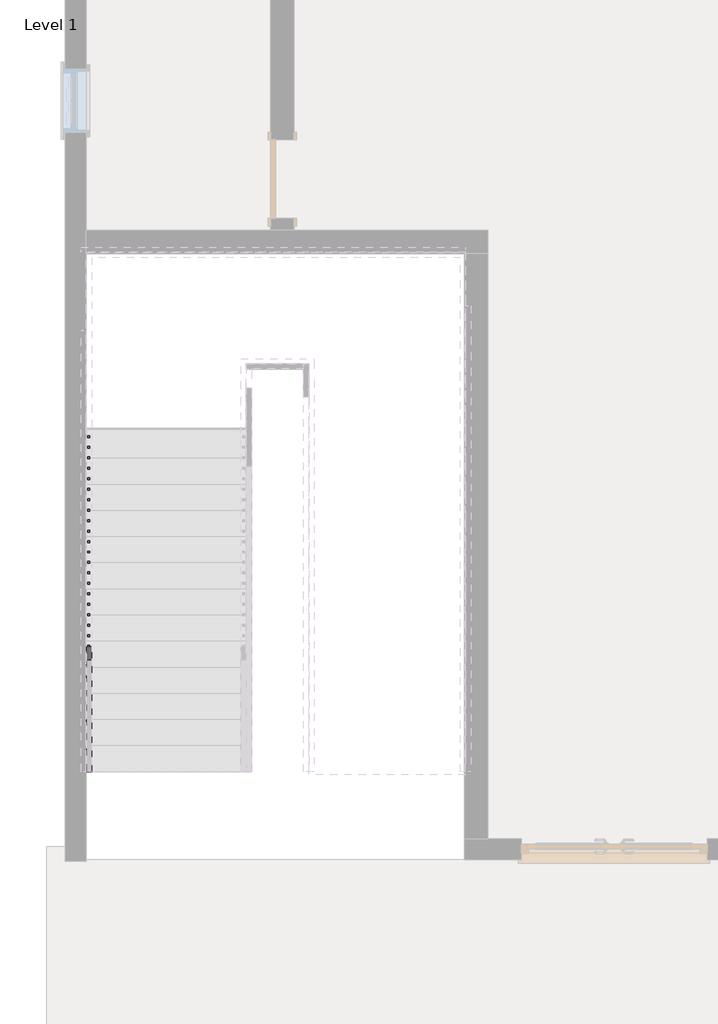
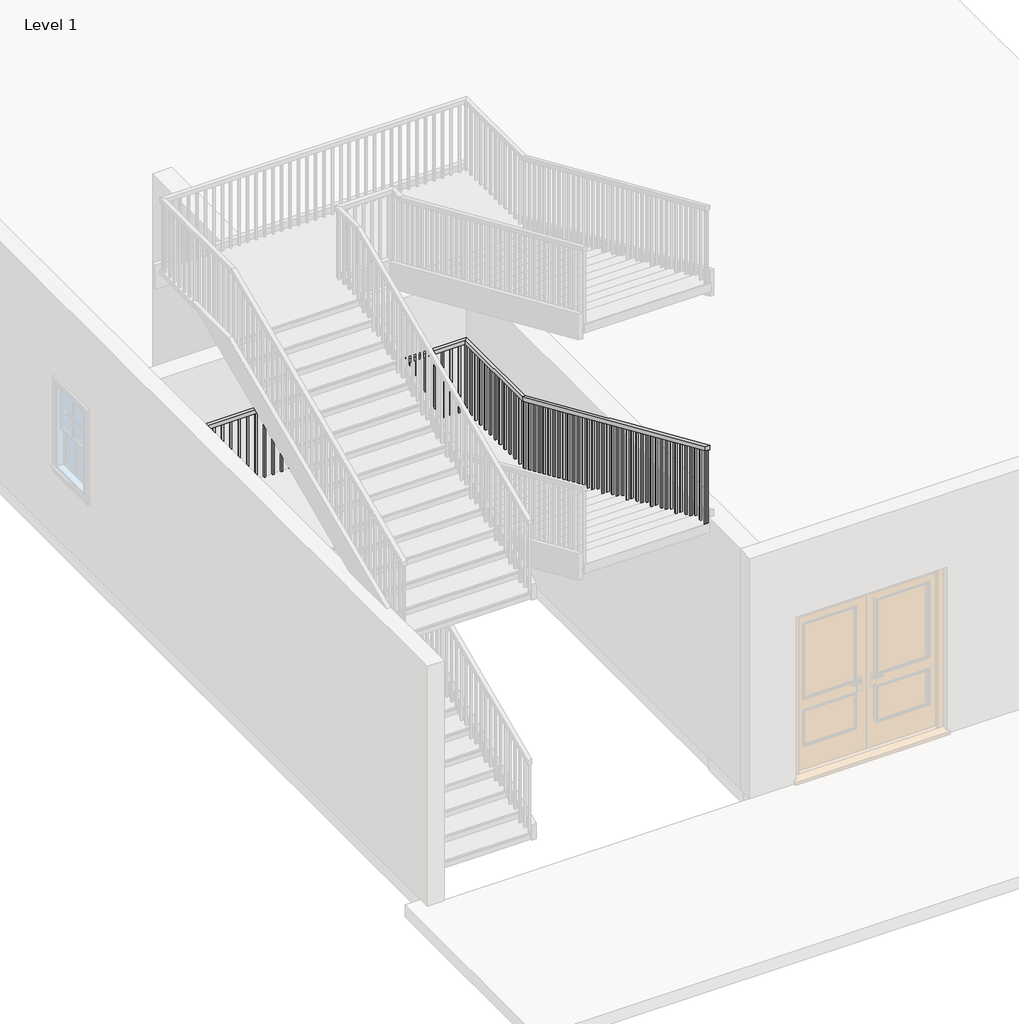
# One storey, part 3 of 6: 1 railing.
"""IFC4 building model written with IfcOpenShell, lengths in millimetres."""

from ifc_helpers import new_model, si_unit, frame, origin, place, context, project, spatial, polyline, outline, extrude, faceted_brep, element, save

model = new_model("IFC4")

# Units and contexts
model_context = context("Model", 3, world=origin())
ifc_project = project(units=[si_unit("LENGTHUNIT", "METRE", prefix="MILLI")], contexts=[model_context])

# Site, building, storey
site = spatial("IfcSite", under=ifc_project)
building = spatial("IfcBuilding", under=site)
storey = spatial("IfcBuildingStorey", under=building, Name="Level 1", Elevation=0.0)

# Railing
placement = place(None, origin())
element("IfcRailing", 1, ObjectType="Handrail - Rectangular", at=placement, inside=storey, context=model_context, shape_type="SolidModel", body=[
    faceted_brep([(-7554.4415084, -6973.0610642, 721.36), (-7554.4415084, -6973.0610642, 665.8599828), (-7503.6415084, -6973.0610642, 665.8599828), (-7503.6415084, -6973.0610642, 721.36), (-7554.4415084, -3417.0610642, 2286.0), (-7554.4415084, -3406.3792071, 2235.2), (-7503.6415084, -3406.3792071, 2235.2), (-7503.6415084, -3417.0610642, 2286.0), (-7554.4415084, -1928.4217109, 2286.0), (-7554.4415084, -1928.4217109, 2235.2), (-7503.6415084, -1979.2217109, 2235.2), (-7503.6415084, -1979.2217109, 2286.0), (-3866.3290366, -1928.4217109, 2286.0), (-3866.3290366, -1928.4217109, 2235.2), (-3917.1290366, -1979.2217109, 2235.2), (-3917.1290366, -1979.2217109, 2286.0), (-3866.3290366, -3163.0610642, 2286.0), (-3866.3290366, -3173.7429214, 2235.2), (-3917.1290366, -3173.7429214, 2235.2), (-3917.1290366, -3163.0610642, 2286.0), (-3866.3290366, -6973.0610642, 3962.4), (-3917.1290366, -6973.0610642, 3962.4), (-3917.1290366, -6973.0610642, 3906.8999828), (-3866.3290366, -6973.0610642, 3906.8999828)], [[[0, 1, 2, 3]], [[1, 0, 4, 5]], [[2, 1, 5, 6]], [[3, 2, 6, 7]], [[0, 3, 7, 4]], [[5, 4, 8, 9]], [[6, 5, 9, 10]], [[7, 6, 10, 11]], [[4, 7, 11, 8]], [[9, 8, 12, 13]], [[10, 9, 13, 14]], [[11, 10, 14, 15]], [[8, 11, 15, 12]], [[13, 12, 16, 17]], [[14, 13, 17, 18]], [[15, 14, 18, 19]], [[12, 15, 19, 16]], [[20, 21, 22, 23]], [[17, 16, 20, 23]], [[18, 17, 23, 22]], [[19, 18, 22, 21]], [[16, 19, 21, 20]]]),
    extrude(outline(polyline([(-6922.6967109, 3884.7396674), (-6922.6967109, 2936.24), (-6941.7467109, 2936.24), (-6941.7467109, 3893.1216674), (-6922.6967109, 3884.7396674)])), frame((-3901.2540366, 0.0, 0.0), z_axis=(1.0, 0.0, 0.0), x_axis=(0.0, 1.0, 0.0)), (0.0, 0.0, 1.0), 19.05),
    extrude(outline(polyline([(-6821.0967109, 3840.0356674), (-6821.0967109, 2936.24), (-6840.1467109, 2936.24), (-6840.1467109, 3848.4176674), (-6821.0967109, 3840.0356674)])), frame((-3901.2540366, 0.0, 0.0), z_axis=(1.0, 0.0, 0.0), x_axis=(0.0, 1.0, 0.0)), (0.0, 0.0, 1.0), 19.05),
    extrude(outline(polyline([(-6719.4967109, 3795.3316674), (-6719.4967109, 2936.24), (-6738.5467109, 2936.24), (-6738.5467109, 3803.7136674), (-6719.4967109, 3795.3316674)])), frame((-3901.2540366, 0.0, 0.0), z_axis=(1.0, 0.0, 0.0), x_axis=(0.0, 1.0, 0.0)), (0.0, 0.0, 1.0), 19.05),
    extrude(outline(polyline([(-6617.8967109, 3750.6276674), (-6617.8967109, 2824.48), (-6636.9467109, 2824.48), (-6636.9467109, 3759.0096674), (-6617.8967109, 3750.6276674)])), frame((-3901.2540366, 0.0, 0.0), z_axis=(1.0, 0.0, 0.0), x_axis=(0.0, 1.0, 0.0)), (0.0, 0.0, 1.0), 19.05),
    extrude(outline(polyline([(-6516.2967109, 3705.9236674), (-6516.2967109, 2824.48), (-6535.3467109, 2824.48), (-6535.3467109, 3714.3056674), (-6516.2967109, 3705.9236674)])), frame((-3901.2540366, 0.0, 0.0), z_axis=(1.0, 0.0, 0.0), x_axis=(0.0, 1.0, 0.0)), (0.0, 0.0, 1.0), 19.05),
    extrude(outline(polyline([(-6414.6967109, 3661.2196674), (-6414.6967109, 2712.72), (-6433.7467109, 2712.72), (-6433.7467109, 3669.6016674), (-6414.6967109, 3661.2196674)])), frame((-3901.2540366, 0.0, 0.0), z_axis=(1.0, 0.0, 0.0), x_axis=(0.0, 1.0, 0.0)), (0.0, 0.0, 1.0), 19.05),
    extrude(outline(polyline([(-6313.0967109, 3616.5156674), (-6313.0967109, 2712.72), (-6332.1467109, 2712.72), (-6332.1467109, 3624.8976674), (-6313.0967109, 3616.5156674)])), frame((-3901.2540366, 0.0, 0.0), z_axis=(1.0, 0.0, 0.0), x_axis=(0.0, 1.0, 0.0)), (0.0, 0.0, 1.0), 19.05),
    extrude(outline(polyline([(-6211.4967109, 3571.8116674), (-6211.4967109, 2712.72), (-6230.5467109, 2712.72), (-6230.5467109, 3580.1936674), (-6211.4967109, 3571.8116674)])), frame((-3901.2540366, 0.0, 0.0), z_axis=(1.0, 0.0, 0.0), x_axis=(0.0, 1.0, 0.0)), (0.0, 0.0, 1.0), 19.05),
    extrude(outline(polyline([(-6109.8967109, 3527.1076674), (-6109.8967109, 2600.96), (-6128.9467109, 2600.96), (-6128.9467109, 3535.4896674), (-6109.8967109, 3527.1076674)])), frame((-3901.2540366, 0.0, 0.0), z_axis=(1.0, 0.0, 0.0), x_axis=(0.0, 1.0, 0.0)), (0.0, 0.0, 1.0), 19.05),
    extrude(outline(polyline([(-6008.2967109, 3482.4036674), (-6008.2967109, 2600.96), (-6027.3467109, 2600.96), (-6027.3467109, 3490.7856674), (-6008.2967109, 3482.4036674)])), frame((-3901.2540366, 0.0, 0.0), z_axis=(1.0, 0.0, 0.0), x_axis=(0.0, 1.0, 0.0)), (0.0, 0.0, 1.0), 19.05),
    extrude(outline(polyline([(-5906.6967109, 3437.6996674), (-5906.6967109, 2489.2), (-5925.7467109, 2489.2), (-5925.7467109, 3446.0816674), (-5906.6967109, 3437.6996674)])), frame((-3901.2540366, 0.0, 0.0), z_axis=(1.0, 0.0, 0.0), x_axis=(0.0, 1.0, 0.0)), (0.0, 0.0, 1.0), 19.05),
    extrude(outline(polyline([(-5805.0967109, 3392.9956674), (-5805.0967109, 2489.2), (-5824.1467109, 2489.2), (-5824.1467109, 3401.3776674), (-5805.0967109, 3392.9956674)])), frame((-3901.2540366, 0.0, 0.0), z_axis=(1.0, 0.0, 0.0), x_axis=(0.0, 1.0, 0.0)), (0.0, 0.0, 1.0), 19.05),
    extrude(outline(polyline([(-5703.4967109, 3348.2916674), (-5703.4967109, 2489.2), (-5722.5467109, 2489.2), (-5722.5467109, 3356.6736674), (-5703.4967109, 3348.2916674)])), frame((-3901.2540366, 0.0, 0.0), z_axis=(1.0, 0.0, 0.0), x_axis=(0.0, 1.0, 0.0)), (0.0, 0.0, 1.0), 19.05),
    extrude(outline(polyline([(-5601.8967109, 3303.5876674), (-5601.8967109, 2377.44), (-5620.9467109, 2377.44), (-5620.9467109, 3311.9696674), (-5601.8967109, 3303.5876674)])), frame((-3901.2540366, 0.0, 0.0), z_axis=(1.0, 0.0, 0.0), x_axis=(0.0, 1.0, 0.0)), (0.0, 0.0, 1.0), 19.05),
    extrude(outline(polyline([(-5500.2967109, 3258.8836674), (-5500.2967109, 2377.44), (-5519.3467109, 2377.44), (-5519.3467109, 3267.2656674), (-5500.2967109, 3258.8836674)])), frame((-3901.2540366, 0.0, 0.0), z_axis=(1.0, 0.0, 0.0), x_axis=(0.0, 1.0, 0.0)), (0.0, 0.0, 1.0), 19.05),
    extrude(outline(polyline([(-5398.6967109, 3214.1796674), (-5398.6967109, 2265.68), (-5417.7467109, 2265.68), (-5417.7467109, 3222.5616674), (-5398.6967109, 3214.1796674)])), frame((-3901.2540366, 0.0, 0.0), z_axis=(1.0, 0.0, 0.0), x_axis=(0.0, 1.0, 0.0)), (0.0, 0.0, 1.0), 19.05),
    extrude(outline(polyline([(-5297.0967109, 3169.4756674), (-5297.0967109, 2265.68), (-5316.1467109, 2265.68), (-5316.1467109, 3177.8576674), (-5297.0967109, 3169.4756674)])), frame((-3901.2540366, 0.0, 0.0), z_axis=(1.0, 0.0, 0.0), x_axis=(0.0, 1.0, 0.0)), (0.0, 0.0, 1.0), 19.05),
    extrude(outline(polyline([(-5195.4967109, 3124.7716674), (-5195.4967109, 2265.68), (-5214.5467109, 2265.68), (-5214.5467109, 3133.1536674), (-5195.4967109, 3124.7716674)])), frame((-3901.2540366, 0.0, 0.0), z_axis=(1.0, 0.0, 0.0), x_axis=(0.0, 1.0, 0.0)), (0.0, 0.0, 1.0), 19.05),
    extrude(outline(polyline([(-5093.8967109, 3080.0676674), (-5093.8967109, 2153.92), (-5112.9467109, 2153.92), (-5112.9467109, 3088.4496674), (-5093.8967109, 3080.0676674)])), frame((-3901.2540366, 0.0, 0.0), z_axis=(1.0, 0.0, 0.0), x_axis=(0.0, 1.0, 0.0)), (0.0, 0.0, 1.0), 19.05),
    extrude(outline(polyline([(-4992.2967109, 3035.3636674), (-4992.2967109, 2153.92), (-5011.3467109, 2153.92), (-5011.3467109, 3043.7456674), (-4992.2967109, 3035.3636674)])), frame((-3901.2540366, 0.0, 0.0), z_axis=(1.0, 0.0, 0.0), x_axis=(0.0, 1.0, 0.0)), (0.0, 0.0, 1.0), 19.05),
    extrude(outline(polyline([(-4890.6967109, 2990.6596674), (-4890.6967109, 2042.16), (-4909.7467109, 2042.16), (-4909.7467109, 2999.0416674), (-4890.6967109, 2990.6596674)])), frame((-3901.2540366, 0.0, 0.0), z_axis=(1.0, 0.0, 0.0), x_axis=(0.0, 1.0, 0.0)), (0.0, 0.0, 1.0), 19.05),
    extrude(outline(polyline([(-4789.0967109, 2945.9556674), (-4789.0967109, 2042.16), (-4808.1467109, 2042.16), (-4808.1467109, 2954.3376674), (-4789.0967109, 2945.9556674)])), frame((-3901.2540366, 0.0, 0.0), z_axis=(1.0, 0.0, 0.0), x_axis=(0.0, 1.0, 0.0)), (0.0, 0.0, 1.0), 19.05),
    extrude(outline(polyline([(-4687.4967109, 2901.2516674), (-4687.4967109, 2042.16), (-4706.5467109, 2042.16), (-4706.5467109, 2909.6336674), (-4687.4967109, 2901.2516674)])), frame((-3901.2540366, 0.0, 0.0), z_axis=(1.0, 0.0, 0.0), x_axis=(0.0, 1.0, 0.0)), (0.0, 0.0, 1.0), 19.05),
    extrude(outline(polyline([(-4585.8967109, 2856.5476674), (-4585.8967109, 1930.4), (-4604.9467109, 1930.4), (-4604.9467109, 2864.9296674), (-4585.8967109, 2856.5476674)])), frame((-3901.2540366, 0.0, 0.0), z_axis=(1.0, 0.0, 0.0), x_axis=(0.0, 1.0, 0.0)), (0.0, 0.0, 1.0), 19.05),
    extrude(outline(polyline([(-4484.2967109, 2811.8436674), (-4484.2967109, 1930.4), (-4503.3467109, 1930.4), (-4503.3467109, 2820.2256674), (-4484.2967109, 2811.8436674)])), frame((-3901.2540366, 0.0, 0.0), z_axis=(1.0, 0.0, 0.0), x_axis=(0.0, 1.0, 0.0)), (0.0, 0.0, 1.0), 19.05),
    extrude(outline(polyline([(-4382.6967109, 2767.1396674), (-4382.6967109, 1818.64), (-4401.7467109, 1818.64), (-4401.7467109, 2775.5216674), (-4382.6967109, 2767.1396674)])), frame((-3901.2540366, 0.0, 0.0), z_axis=(1.0, 0.0, 0.0), x_axis=(0.0, 1.0, 0.0)), (0.0, 0.0, 1.0), 19.05),
    extrude(outline(polyline([(-4281.0967109, 2722.4356674), (-4281.0967109, 1818.64), (-4300.1467109, 1818.64), (-4300.1467109, 2730.8176674), (-4281.0967109, 2722.4356674)])), frame((-3901.2540366, 0.0, 0.0), z_axis=(1.0, 0.0, 0.0), x_axis=(0.0, 1.0, 0.0)), (0.0, 0.0, 1.0), 19.05),
    extrude(outline(polyline([(-4179.4967109, 2677.7316674), (-4179.4967109, 1818.64), (-4198.5467109, 1818.64), (-4198.5467109, 2686.1136674), (-4179.4967109, 2677.7316674)])), frame((-3901.2540366, 0.0, 0.0), z_axis=(1.0, 0.0, 0.0), x_axis=(0.0, 1.0, 0.0)), (0.0, 0.0, 1.0), 19.05),
    extrude(outline(polyline([(-4077.8967109, 2633.0276674), (-4077.8967109, 1706.88), (-4096.9467109, 1706.88), (-4096.9467109, 2641.4096674), (-4077.8967109, 2633.0276674)])), frame((-3901.2540366, 0.0, 0.0), z_axis=(1.0, 0.0, 0.0), x_axis=(0.0, 1.0, 0.0)), (0.0, 0.0, 1.0), 19.05),
    extrude(outline(polyline([(-3976.2967109, 2588.3236674), (-3976.2967109, 1706.88), (-3995.3467109, 1706.88), (-3995.3467109, 2596.7056674), (-3976.2967109, 2588.3236674)])), frame((-3901.2540366, 0.0, 0.0), z_axis=(1.0, 0.0, 0.0), x_axis=(0.0, 1.0, 0.0)), (0.0, 0.0, 1.0), 19.05),
    extrude(outline(polyline([(-3874.6967109, 2543.6196674), (-3874.6967109, 1595.12), (-3893.7467109, 1595.12), (-3893.7467109, 2552.0016674), (-3874.6967109, 2543.6196674)])), frame((-3901.2540366, 0.0, 0.0), z_axis=(1.0, 0.0, 0.0), x_axis=(0.0, 1.0, 0.0)), (0.0, 0.0, 1.0), 19.05),
    extrude(outline(polyline([(-3773.0967109, 2498.9156674), (-3773.0967109, 1595.12), (-3792.1467109, 1595.12), (-3792.1467109, 2507.2976674), (-3773.0967109, 2498.9156674)])), frame((-3901.2540366, 0.0, 0.0), z_axis=(1.0, 0.0, 0.0), x_axis=(0.0, 1.0, 0.0)), (0.0, 0.0, 1.0), 19.05),
    extrude(outline(polyline([(-3671.4967109, 2454.2116674), (-3671.4967109, 1595.12), (-3690.5467109, 1595.12), (-3690.5467109, 2462.5936674), (-3671.4967109, 2454.2116674)])), frame((-3901.2540366, 0.0, 0.0), z_axis=(1.0, 0.0, 0.0), x_axis=(0.0, 1.0, 0.0)), (0.0, 0.0, 1.0), 19.05),
    extrude(outline(polyline([(-3569.8967109, 2409.5076674), (-3569.8967109, 1483.36), (-3588.9467109, 1483.36), (-3588.9467109, 2417.8896674), (-3569.8967109, 2409.5076674)])), frame((-3901.2540366, 0.0, 0.0), z_axis=(1.0, 0.0, 0.0), x_axis=(0.0, 1.0, 0.0)), (0.0, 0.0, 1.0), 19.05),
    extrude(outline(polyline([(-3468.2967109, 2364.8036674), (-3468.2967109, 1483.36), (-3487.3467109, 1483.36), (-3487.3467109, 2373.1856674), (-3468.2967109, 2364.8036674)])), frame((-3901.2540366, 0.0, 0.0), z_axis=(1.0, 0.0, 0.0), x_axis=(0.0, 1.0, 0.0)), (0.0, 0.0, 1.0), 19.05),
    extrude(outline(polyline([(-3366.6967109, 2320.0996674), (-3366.6967109, 1371.6), (-3385.7467109, 1371.6), (-3385.7467109, 2328.4816674), (-3366.6967109, 2320.0996674)])), frame((-3901.2540366, 0.0, 0.0), z_axis=(1.0, 0.0, 0.0), x_axis=(0.0, 1.0, 0.0)), (0.0, 0.0, 1.0), 19.05),
    extrude(outline(polyline([(-3265.0967109, 2275.3956674), (-3265.0967109, 1371.6), (-3284.1467109, 1371.6), (-3284.1467109, 2283.7776674), (-3265.0967109, 2275.3956674)])), frame((-3901.2540366, 0.0, 0.0), z_axis=(1.0, 0.0, 0.0), x_axis=(0.0, 1.0, 0.0)), (0.0, 0.0, 1.0), 19.05),
    extrude(outline(polyline([(-3163.4967109, 2230.6916674), (-3163.4967109, 1371.6), (-3182.5467109, 1371.6), (-3182.5467109, 2239.0736674), (-3163.4967109, 2230.6916674)])), frame((-3901.2540366, 0.0, 0.0), z_axis=(1.0, 0.0, 0.0), x_axis=(0.0, 1.0, 0.0)), (0.0, 0.0, 1.0), 19.05),
    extrude(outline(polyline([(-3882.2040366, -3061.8967109), (-3882.2040366, -3080.9467109), (-3901.2540366, -3080.9467109), (-3901.2540366, -3061.8967109), (-3882.2040366, -3061.8967109)])), frame((0.0, 0.0, 1371.6), z_axis=(0.0, 0.0, 1.0), x_axis=(1.0, 0.0, 0.0)), (0.0, 0.0, 1.0), 863.6),
    extrude(outline(polyline([(-3882.2040366, -2960.2967109), (-3882.2040366, -2979.3467109), (-3901.2540366, -2979.3467109), (-3901.2540366, -2960.2967109), (-3882.2040366, -2960.2967109)])), frame((0.0, 0.0, 1371.6), z_axis=(0.0, 0.0, 1.0), x_axis=(1.0, 0.0, 0.0)), (0.0, 0.0, 1.0), 863.6),
    extrude(outline(polyline([(-3882.2040366, -2858.6967109), (-3882.2040366, -2877.7467109), (-3901.2540366, -2877.7467109), (-3901.2540366, -2858.6967109), (-3882.2040366, -2858.6967109)])), frame((0.0, 0.0, 1371.6), z_axis=(0.0, 0.0, 1.0), x_axis=(1.0, 0.0, 0.0)), (0.0, 0.0, 1.0), 863.6),
    extrude(outline(polyline([(-3882.2040366, -2757.0967109), (-3882.2040366, -2776.1467109), (-3901.2540366, -2776.1467109), (-3901.2540366, -2757.0967109), (-3882.2040366, -2757.0967109)])), frame((0.0, 0.0, 1371.6), z_axis=(0.0, 0.0, 1.0), x_axis=(1.0, 0.0, 0.0)), (0.0, 0.0, 1.0), 863.6),
    extrude(outline(polyline([(-3882.2040366, -2655.4967109), (-3882.2040366, -2674.5467109), (-3901.2540366, -2674.5467109), (-3901.2540366, -2655.4967109), (-3882.2040366, -2655.4967109)])), frame((0.0, 0.0, 1371.6), z_axis=(0.0, 0.0, 1.0), x_axis=(1.0, 0.0, 0.0)), (0.0, 0.0, 1.0), 863.6),
    extrude(outline(polyline([(-3882.2040366, -2553.8967109), (-3882.2040366, -2572.9467109), (-3901.2540366, -2572.9467109), (-3901.2540366, -2553.8967109), (-3882.2040366, -2553.8967109)])), frame((0.0, 0.0, 1371.6), z_axis=(0.0, 0.0, 1.0), x_axis=(1.0, 0.0, 0.0)), (0.0, 0.0, 1.0), 863.6),
    extrude(outline(polyline([(-3882.2040366, -2452.2967109), (-3882.2040366, -2471.3467109), (-3901.2540366, -2471.3467109), (-3901.2540366, -2452.2967109), (-3882.2040366, -2452.2967109)])), frame((0.0, 0.0, 1371.6), z_axis=(0.0, 0.0, 1.0), x_axis=(1.0, 0.0, 0.0)), (0.0, 0.0, 1.0), 863.6),
    extrude(outline(polyline([(-3882.2040366, -2350.6967109), (-3882.2040366, -2369.7467109), (-3901.2540366, -2369.7467109), (-3901.2540366, -2350.6967109), (-3882.2040366, -2350.6967109)])), frame((0.0, 0.0, 1371.6), z_axis=(0.0, 0.0, 1.0), x_axis=(1.0, 0.0, 0.0)), (0.0, 0.0, 1.0), 863.6),
    extrude(outline(polyline([(-3882.2040366, -2249.0967109), (-3882.2040366, -2268.1467109), (-3901.2540366, -2268.1467109), (-3901.2540366, -2249.0967109), (-3882.2040366, -2249.0967109)])), frame((0.0, 0.0, 1371.6), z_axis=(0.0, 0.0, 1.0), x_axis=(1.0, 0.0, 0.0)), (0.0, 0.0, 1.0), 863.6),
    extrude(outline(polyline([(-3882.2040366, -2147.4967109), (-3882.2040366, -2166.5467109), (-3901.2540366, -2166.5467109), (-3901.2540366, -2147.4967109), (-3882.2040366, -2147.4967109)])), frame((0.0, 0.0, 1371.6), z_axis=(0.0, 0.0, 1.0), x_axis=(1.0, 0.0, 0.0)), (0.0, 0.0, 1.0), 863.6),
    extrude(outline(polyline([(-3882.2040366, -2045.8967109), (-3882.2040366, -2064.9467109), (-3901.2540366, -2064.9467109), (-3901.2540366, -2045.8967109), (-3882.2040366, -2045.8967109)])), frame((0.0, 0.0, 1371.6), z_axis=(0.0, 0.0, 1.0), x_axis=(1.0, 0.0, 0.0)), (0.0, 0.0, 1.0), 863.6),
    extrude(outline(polyline([(-3982.5665084, -1944.2967109), (-3963.5165084, -1944.2967109), (-3963.5165084, -1963.3467109), (-3982.5665084, -1963.3467109), (-3982.5665084, -1944.2967109)])), frame((0.0, 0.0, 1371.6), z_axis=(0.0, 0.0, 1.0), x_axis=(1.0, 0.0, 0.0)), (0.0, 0.0, 1.0), 863.6),
    extrude(outline(polyline([(-4084.1665084, -1944.2967109), (-4065.1165084, -1944.2967109), (-4065.1165084, -1963.3467109), (-4084.1665084, -1963.3467109), (-4084.1665084, -1944.2967109)])), frame((0.0, 0.0, 1371.6), z_axis=(0.0, 0.0, 1.0), x_axis=(1.0, 0.0, 0.0)), (0.0, 0.0, 1.0), 863.6),
    extrude(outline(polyline([(-4185.7665084, -1944.2967109), (-4166.7165084, -1944.2967109), (-4166.7165084, -1963.3467109), (-4185.7665084, -1963.3467109), (-4185.7665084, -1944.2967109)])), frame((0.0, 0.0, 1371.6), z_axis=(0.0, 0.0, 1.0), x_axis=(1.0, 0.0, 0.0)), (0.0, 0.0, 1.0), 863.6),
    extrude(outline(polyline([(-4287.3665084, -1944.2967109), (-4268.3165084, -1944.2967109), (-4268.3165084, -1963.3467109), (-4287.3665084, -1963.3467109), (-4287.3665084, -1944.2967109)])), frame((0.0, 0.0, 1371.6), z_axis=(0.0, 0.0, 1.0), x_axis=(1.0, 0.0, 0.0)), (0.0, 0.0, 1.0), 863.6),
    extrude(outline(polyline([(-4388.9665084, -1944.2967109), (-4369.9165084, -1944.2967109), (-4369.9165084, -1963.3467109), (-4388.9665084, -1963.3467109), (-4388.9665084, -1944.2967109)])), frame((0.0, 0.0, 1371.6), z_axis=(0.0, 0.0, 1.0), x_axis=(1.0, 0.0, 0.0)), (0.0, 0.0, 1.0), 863.6),
    extrude(outline(polyline([(-4490.5665084, -1944.2967109), (-4471.5165084, -1944.2967109), (-4471.5165084, -1963.3467109), (-4490.5665084, -1963.3467109), (-4490.5665084, -1944.2967109)])), frame((0.0, 0.0, 1371.6), z_axis=(0.0, 0.0, 1.0), x_axis=(1.0, 0.0, 0.0)), (0.0, 0.0, 1.0), 863.6),
    extrude(outline(polyline([(-4592.1665084, -1944.2967109), (-4573.1165084, -1944.2967109), (-4573.1165084, -1963.3467109), (-4592.1665084, -1963.3467109), (-4592.1665084, -1944.2967109)])), frame((0.0, 0.0, 1371.6), z_axis=(0.0, 0.0, 1.0), x_axis=(1.0, 0.0, 0.0)), (0.0, 0.0, 1.0), 863.6),
    extrude(outline(polyline([(-4693.7665084, -1944.2967109), (-4674.7165084, -1944.2967109), (-4674.7165084, -1963.3467109), (-4693.7665084, -1963.3467109), (-4693.7665084, -1944.2967109)])), frame((0.0, 0.0, 1371.6), z_axis=(0.0, 0.0, 1.0), x_axis=(1.0, 0.0, 0.0)), (0.0, 0.0, 1.0), 863.6),
    extrude(outline(polyline([(-4795.3665084, -1944.2967109), (-4776.3165084, -1944.2967109), (-4776.3165084, -1963.3467109), (-4795.3665084, -1963.3467109), (-4795.3665084, -1944.2967109)])), frame((0.0, 0.0, 1371.6), z_axis=(0.0, 0.0, 1.0), x_axis=(1.0, 0.0, 0.0)), (0.0, 0.0, 1.0), 863.6),
    extrude(outline(polyline([(-4896.9665084, -1944.2967109), (-4877.9165084, -1944.2967109), (-4877.9165084, -1963.3467109), (-4896.9665084, -1963.3467109), (-4896.9665084, -1944.2967109)])), frame((0.0, 0.0, 1371.6), z_axis=(0.0, 0.0, 1.0), x_axis=(1.0, 0.0, 0.0)), (0.0, 0.0, 1.0), 863.6),
    extrude(outline(polyline([(-4998.5665084, -1944.2967109), (-4979.5165084, -1944.2967109), (-4979.5165084, -1963.3467109), (-4998.5665084, -1963.3467109), (-4998.5665084, -1944.2967109)])), frame((0.0, 0.0, 1371.6), z_axis=(0.0, 0.0, 1.0), x_axis=(1.0, 0.0, 0.0)), (0.0, 0.0, 1.0), 863.6),
    extrude(outline(polyline([(-5100.1665084, -1944.2967109), (-5081.1165084, -1944.2967109), (-5081.1165084, -1963.3467109), (-5100.1665084, -1963.3467109), (-5100.1665084, -1944.2967109)])), frame((0.0, 0.0, 1371.6), z_axis=(0.0, 0.0, 1.0), x_axis=(1.0, 0.0, 0.0)), (0.0, 0.0, 1.0), 863.6),
    extrude(outline(polyline([(-5201.7665084, -1944.2967109), (-5182.7165084, -1944.2967109), (-5182.7165084, -1963.3467109), (-5201.7665084, -1963.3467109), (-5201.7665084, -1944.2967109)])), frame((0.0, 0.0, 1371.6), z_axis=(0.0, 0.0, 1.0), x_axis=(1.0, 0.0, 0.0)), (0.0, 0.0, 1.0), 863.6),
    extrude(outline(polyline([(-5303.3665084, -1944.2967109), (-5284.3165084, -1944.2967109), (-5284.3165084, -1963.3467109), (-5303.3665084, -1963.3467109), (-5303.3665084, -1944.2967109)])), frame((0.0, 0.0, 1371.6), z_axis=(0.0, 0.0, 1.0), x_axis=(1.0, 0.0, 0.0)), (0.0, 0.0, 1.0), 863.6),
    extrude(outline(polyline([(-5404.9665084, -1944.2967109), (-5385.9165084, -1944.2967109), (-5385.9165084, -1963.3467109), (-5404.9665084, -1963.3467109), (-5404.9665084, -1944.2967109)])), frame((0.0, 0.0, 1371.6), z_axis=(0.0, 0.0, 1.0), x_axis=(1.0, 0.0, 0.0)), (0.0, 0.0, 1.0), 863.6),
    extrude(outline(polyline([(-5506.5665084, -1944.2967109), (-5487.5165084, -1944.2967109), (-5487.5165084, -1963.3467109), (-5506.5665084, -1963.3467109), (-5506.5665084, -1944.2967109)])), frame((0.0, 0.0, 1371.6), z_axis=(0.0, 0.0, 1.0), x_axis=(1.0, 0.0, 0.0)), (0.0, 0.0, 1.0), 863.6),
    extrude(outline(polyline([(-5608.1665084, -1944.2967109), (-5589.1165084, -1944.2967109), (-5589.1165084, -1963.3467109), (-5608.1665084, -1963.3467109), (-5608.1665084, -1944.2967109)])), frame((0.0, 0.0, 1371.6), z_axis=(0.0, 0.0, 1.0), x_axis=(1.0, 0.0, 0.0)), (0.0, 0.0, 1.0), 863.6),
    extrude(outline(polyline([(-5709.7665084, -1944.2967109), (-5690.7165084, -1944.2967109), (-5690.7165084, -1963.3467109), (-5709.7665084, -1963.3467109), (-5709.7665084, -1944.2967109)])), frame((0.0, 0.0, 1371.6), z_axis=(0.0, 0.0, 1.0), x_axis=(1.0, 0.0, 0.0)), (0.0, 0.0, 1.0), 863.6),
    extrude(outline(polyline([(-5811.3665084, -1944.2967109), (-5792.3165084, -1944.2967109), (-5792.3165084, -1963.3467109), (-5811.3665084, -1963.3467109), (-5811.3665084, -1944.2967109)])), frame((0.0, 0.0, 1371.6), z_axis=(0.0, 0.0, 1.0), x_axis=(1.0, 0.0, 0.0)), (0.0, 0.0, 1.0), 863.6),
    extrude(outline(polyline([(-5912.9665084, -1944.2967109), (-5893.9165084, -1944.2967109), (-5893.9165084, -1963.3467109), (-5912.9665084, -1963.3467109), (-5912.9665084, -1944.2967109)])), frame((0.0, 0.0, 1371.6), z_axis=(0.0, 0.0, 1.0), x_axis=(1.0, 0.0, 0.0)), (0.0, 0.0, 1.0), 863.6),
    extrude(outline(polyline([(-6014.5665084, -1944.2967109), (-5995.5165084, -1944.2967109), (-5995.5165084, -1963.3467109), (-6014.5665084, -1963.3467109), (-6014.5665084, -1944.2967109)])), frame((0.0, 0.0, 1371.6), z_axis=(0.0, 0.0, 1.0), x_axis=(1.0, 0.0, 0.0)), (0.0, 0.0, 1.0), 863.6),
    extrude(outline(polyline([(-6116.1665084, -1944.2967109), (-6097.1165084, -1944.2967109), (-6097.1165084, -1963.3467109), (-6116.1665084, -1963.3467109), (-6116.1665084, -1944.2967109)])), frame((0.0, 0.0, 1371.6), z_axis=(0.0, 0.0, 1.0), x_axis=(1.0, 0.0, 0.0)), (0.0, 0.0, 1.0), 863.6),
    extrude(outline(polyline([(-6217.7665084, -1944.2967109), (-6198.7165084, -1944.2967109), (-6198.7165084, -1963.3467109), (-6217.7665084, -1963.3467109), (-6217.7665084, -1944.2967109)])), frame((0.0, 0.0, 1371.6), z_axis=(0.0, 0.0, 1.0), x_axis=(1.0, 0.0, 0.0)), (0.0, 0.0, 1.0), 863.6),
    extrude(outline(polyline([(-6319.3665084, -1944.2967109), (-6300.3165084, -1944.2967109), (-6300.3165084, -1963.3467109), (-6319.3665084, -1963.3467109), (-6319.3665084, -1944.2967109)])), frame((0.0, 0.0, 1371.6), z_axis=(0.0, 0.0, 1.0), x_axis=(1.0, 0.0, 0.0)), (0.0, 0.0, 1.0), 863.6),
    extrude(outline(polyline([(-6420.9665084, -1944.2967109), (-6401.9165084, -1944.2967109), (-6401.9165084, -1963.3467109), (-6420.9665084, -1963.3467109), (-6420.9665084, -1944.2967109)])), frame((0.0, 0.0, 1371.6), z_axis=(0.0, 0.0, 1.0), x_axis=(1.0, 0.0, 0.0)), (0.0, 0.0, 1.0), 863.6),
    extrude(outline(polyline([(-6522.5665084, -1944.2967109), (-6503.5165084, -1944.2967109), (-6503.5165084, -1963.3467109), (-6522.5665084, -1963.3467109), (-6522.5665084, -1944.2967109)])), frame((0.0, 0.0, 1371.6), z_axis=(0.0, 0.0, 1.0), x_axis=(1.0, 0.0, 0.0)), (0.0, 0.0, 1.0), 863.6),
    extrude(outline(polyline([(-6624.1665084, -1944.2967109), (-6605.1165084, -1944.2967109), (-6605.1165084, -1963.3467109), (-6624.1665084, -1963.3467109), (-6624.1665084, -1944.2967109)])), frame((0.0, 0.0, 1371.6), z_axis=(0.0, 0.0, 1.0), x_axis=(1.0, 0.0, 0.0)), (0.0, 0.0, 1.0), 863.6),
    extrude(outline(polyline([(-6725.7665084, -1944.2967109), (-6706.7165084, -1944.2967109), (-6706.7165084, -1963.3467109), (-6725.7665084, -1963.3467109), (-6725.7665084, -1944.2967109)])), frame((0.0, 0.0, 1371.6), z_axis=(0.0, 0.0, 1.0), x_axis=(1.0, 0.0, 0.0)), (0.0, 0.0, 1.0), 863.6),
    extrude(outline(polyline([(-6827.3665084, -1944.2967109), (-6808.3165084, -1944.2967109), (-6808.3165084, -1963.3467109), (-6827.3665084, -1963.3467109), (-6827.3665084, -1944.2967109)])), frame((0.0, 0.0, 1371.6), z_axis=(0.0, 0.0, 1.0), x_axis=(1.0, 0.0, 0.0)), (0.0, 0.0, 1.0), 863.6),
    extrude(outline(polyline([(-6928.9665084, -1944.2967109), (-6909.9165084, -1944.2967109), (-6909.9165084, -1963.3467109), (-6928.9665084, -1963.3467109), (-6928.9665084, -1944.2967109)])), frame((0.0, 0.0, 1371.6), z_axis=(0.0, 0.0, 1.0), x_axis=(1.0, 0.0, 0.0)), (0.0, 0.0, 1.0), 863.6),
    extrude(outline(polyline([(-7030.5665084, -1944.2967109), (-7011.5165084, -1944.2967109), (-7011.5165084, -1963.3467109), (-7030.5665084, -1963.3467109), (-7030.5665084, -1944.2967109)])), frame((0.0, 0.0, 1371.6), z_axis=(0.0, 0.0, 1.0), x_axis=(1.0, 0.0, 0.0)), (0.0, 0.0, 1.0), 863.6),
    extrude(outline(polyline([(-7132.1665084, -1944.2967109), (-7113.1165084, -1944.2967109), (-7113.1165084, -1963.3467109), (-7132.1665084, -1963.3467109), (-7132.1665084, -1944.2967109)])), frame((0.0, 0.0, 1371.6), z_axis=(0.0, 0.0, 1.0), x_axis=(1.0, 0.0, 0.0)), (0.0, 0.0, 1.0), 863.6),
    extrude(outline(polyline([(-7233.7665084, -1944.2967109), (-7214.7165084, -1944.2967109), (-7214.7165084, -1963.3467109), (-7233.7665084, -1963.3467109), (-7233.7665084, -1944.2967109)])), frame((0.0, 0.0, 1371.6), z_axis=(0.0, 0.0, 1.0), x_axis=(1.0, 0.0, 0.0)), (0.0, 0.0, 1.0), 863.6),
    extrude(outline(polyline([(-7335.3665084, -1944.2967109), (-7316.3165084, -1944.2967109), (-7316.3165084, -1963.3467109), (-7335.3665084, -1963.3467109), (-7335.3665084, -1944.2967109)])), frame((0.0, 0.0, 1371.6), z_axis=(0.0, 0.0, 1.0), x_axis=(1.0, 0.0, 0.0)), (0.0, 0.0, 1.0), 863.6),
    extrude(outline(polyline([(-7436.9665084, -1944.2967109), (-7417.9165084, -1944.2967109), (-7417.9165084, -1963.3467109), (-7436.9665084, -1963.3467109), (-7436.9665084, -1944.2967109)])), frame((0.0, 0.0, 1371.6), z_axis=(0.0, 0.0, 1.0), x_axis=(1.0, 0.0, 0.0)), (0.0, 0.0, 1.0), 863.6),
    extrude(outline(polyline([(-7538.5665084, -2004.1860642), (-7538.5665084, -1985.1360642), (-7519.5165084, -1985.1360642), (-7519.5165084, -2004.1860642), (-7538.5665084, -2004.1860642)])), frame((0.0, 0.0, 1371.6), z_axis=(0.0, 0.0, 1.0), x_axis=(1.0, 0.0, 0.0)), (0.0, 0.0, 1.0), 863.6),
    extrude(outline(polyline([(-7538.5665084, -2105.7860642), (-7538.5665084, -2086.7360642), (-7519.5165084, -2086.7360642), (-7519.5165084, -2105.7860642), (-7538.5665084, -2105.7860642)])), frame((0.0, 0.0, 1371.6), z_axis=(0.0, 0.0, 1.0), x_axis=(1.0, 0.0, 0.0)), (0.0, 0.0, 1.0), 863.6),
    extrude(outline(polyline([(-7538.5665084, -2207.3860642), (-7538.5665084, -2188.3360642), (-7519.5165084, -2188.3360642), (-7519.5165084, -2207.3860642), (-7538.5665084, -2207.3860642)])), frame((0.0, 0.0, 1371.6), z_axis=(0.0, 0.0, 1.0), x_axis=(1.0, 0.0, 0.0)), (0.0, 0.0, 1.0), 863.6),
    extrude(outline(polyline([(-7538.5665084, -2308.9860642), (-7538.5665084, -2289.9360642), (-7519.5165084, -2289.9360642), (-7519.5165084, -2308.9860642), (-7538.5665084, -2308.9860642)])), frame((0.0, 0.0, 1371.6), z_axis=(0.0, 0.0, 1.0), x_axis=(1.0, 0.0, 0.0)), (0.0, 0.0, 1.0), 863.6),
    extrude(outline(polyline([(-7538.5665084, -2410.5860642), (-7538.5665084, -2391.5360642), (-7519.5165084, -2391.5360642), (-7519.5165084, -2410.5860642), (-7538.5665084, -2410.5860642)])), frame((0.0, 0.0, 1371.6), z_axis=(0.0, 0.0, 1.0), x_axis=(1.0, 0.0, 0.0)), (0.0, 0.0, 1.0), 863.6),
    extrude(outline(polyline([(-7538.5665084, -2512.1860642), (-7538.5665084, -2493.1360642), (-7519.5165084, -2493.1360642), (-7519.5165084, -2512.1860642), (-7538.5665084, -2512.1860642)])), frame((0.0, 0.0, 1371.6), z_axis=(0.0, 0.0, 1.0), x_axis=(1.0, 0.0, 0.0)), (0.0, 0.0, 1.0), 863.6),
    extrude(outline(polyline([(-7538.5665084, -2613.7860642), (-7538.5665084, -2594.7360642), (-7519.5165084, -2594.7360642), (-7519.5165084, -2613.7860642), (-7538.5665084, -2613.7860642)])), frame((0.0, 0.0, 1371.6), z_axis=(0.0, 0.0, 1.0), x_axis=(1.0, 0.0, 0.0)), (0.0, 0.0, 1.0), 863.6),
    extrude(outline(polyline([(-7538.5665084, -2715.3860642), (-7538.5665084, -2696.3360642), (-7519.5165084, -2696.3360642), (-7519.5165084, -2715.3860642), (-7538.5665084, -2715.3860642)])), frame((0.0, 0.0, 1371.6), z_axis=(0.0, 0.0, 1.0), x_axis=(1.0, 0.0, 0.0)), (0.0, 0.0, 1.0), 863.6),
    extrude(outline(polyline([(-7538.5665084, -2816.9860642), (-7538.5665084, -2797.9360642), (-7519.5165084, -2797.9360642), (-7519.5165084, -2816.9860642), (-7538.5665084, -2816.9860642)])), frame((0.0, 0.0, 1371.6), z_axis=(0.0, 0.0, 1.0), x_axis=(1.0, 0.0, 0.0)), (0.0, 0.0, 1.0), 863.6),
    extrude(outline(polyline([(-7538.5665084, -2918.5860642), (-7538.5665084, -2899.5360642), (-7519.5165084, -2899.5360642), (-7519.5165084, -2918.5860642), (-7538.5665084, -2918.5860642)])), frame((0.0, 0.0, 1371.6), z_axis=(0.0, 0.0, 1.0), x_axis=(1.0, 0.0, 0.0)), (0.0, 0.0, 1.0), 863.6),
    extrude(outline(polyline([(-7538.5665084, -3020.1860642), (-7538.5665084, -3001.1360642), (-7519.5165084, -3001.1360642), (-7519.5165084, -3020.1860642), (-7538.5665084, -3020.1860642)])), frame((0.0, 0.0, 1371.6), z_axis=(0.0, 0.0, 1.0), x_axis=(1.0, 0.0, 0.0)), (0.0, 0.0, 1.0), 863.6),
    extrude(outline(polyline([(-7538.5665084, -3121.7860642), (-7538.5665084, -3102.7360642), (-7519.5165084, -3102.7360642), (-7519.5165084, -3121.7860642), (-7538.5665084, -3121.7860642)])), frame((0.0, 0.0, 1371.6), z_axis=(0.0, 0.0, 1.0), x_axis=(1.0, 0.0, 0.0)), (0.0, 0.0, 1.0), 863.6),
    extrude(outline(polyline([(-7538.5665084, -3223.3860642), (-7538.5665084, -3204.3360642), (-7519.5165084, -3204.3360642), (-7519.5165084, -3223.3860642), (-7538.5665084, -3223.3860642)])), frame((0.0, 0.0, 1371.6), z_axis=(0.0, 0.0, 1.0), x_axis=(1.0, 0.0, 0.0)), (0.0, 0.0, 1.0), 863.6),
    extrude(outline(polyline([(-7538.5665084, -3324.9860642), (-7538.5665084, -3305.9360642), (-7519.5165084, -3305.9360642), (-7519.5165084, -3324.9860642), (-7538.5665084, -3324.9860642)])), frame((0.0, 0.0, 1371.6), z_axis=(0.0, 0.0, 1.0), x_axis=(1.0, 0.0, 0.0)), (0.0, 0.0, 1.0), 863.6),
    extrude(outline(polyline([(-3407.5360642, 2234.6909828), (-3407.5360642, 1371.6), (-3426.5860642, 1371.6), (-3426.5860642, 2226.3089828), (-3407.5360642, 2234.6909828)])), frame((-7538.5665084, 0.0, 0.0), z_axis=(1.0, 0.0, 0.0), x_axis=(0.0, 1.0, 0.0)), (0.0, 0.0, 1.0), 19.05),
    extrude(outline(polyline([(-3509.1360642, 2189.9869828), (-3509.1360642, 1259.84), (-3528.1860642, 1259.84), (-3528.1860642, 2181.6049828), (-3509.1360642, 2189.9869828)])), frame((-7538.5665084, 0.0, 0.0), z_axis=(1.0, 0.0, 0.0), x_axis=(0.0, 1.0, 0.0)), (0.0, 0.0, 1.0), 19.05),
    extrude(outline(polyline([(-3610.7360642, 2145.2829828), (-3610.7360642, 1259.84), (-3629.7860642, 1259.84), (-3629.7860642, 2136.9009828), (-3610.7360642, 2145.2829828)])), frame((-7538.5665084, 0.0, 0.0), z_axis=(1.0, 0.0, 0.0), x_axis=(0.0, 1.0, 0.0)), (0.0, 0.0, 1.0), 19.05),
    extrude(outline(polyline([(-3712.3360642, 2100.5789828), (-3712.3360642, 1148.08), (-3731.3860642, 1148.08), (-3731.3860642, 2092.1969828), (-3712.3360642, 2100.5789828)])), frame((-7538.5665084, 0.0, 0.0), z_axis=(1.0, 0.0, 0.0), x_axis=(0.0, 1.0, 0.0)), (0.0, 0.0, 1.0), 19.05),
    extrude(outline(polyline([(-3813.9360642, 2055.8749828), (-3813.9360642, 1148.08), (-3832.9860642, 1148.08), (-3832.9860642, 2047.4929828), (-3813.9360642, 2055.8749828)])), frame((-7538.5665084, 0.0, 0.0), z_axis=(1.0, 0.0, 0.0), x_axis=(0.0, 1.0, 0.0)), (0.0, 0.0, 1.0), 19.05),
    extrude(outline(polyline([(-3915.5360642, 2011.1709828), (-3915.5360642, 1148.08), (-3934.5860642, 1148.08), (-3934.5860642, 2002.7889828), (-3915.5360642, 2011.1709828)])), frame((-7538.5665084, 0.0, 0.0), z_axis=(1.0, 0.0, 0.0), x_axis=(0.0, 1.0, 0.0)), (0.0, 0.0, 1.0), 19.05),
    extrude(outline(polyline([(-4017.1360642, 1966.4669828), (-4017.1360642, 1036.32), (-4036.1860642, 1036.32), (-4036.1860642, 1958.0849828), (-4017.1360642, 1966.4669828)])), frame((-7538.5665084, 0.0, 0.0), z_axis=(1.0, 0.0, 0.0), x_axis=(0.0, 1.0, 0.0)), (0.0, 0.0, 1.0), 19.05),
    extrude(outline(polyline([(-4118.7360642, 1921.7629828), (-4118.7360642, 1036.32), (-4137.7860642, 1036.32), (-4137.7860642, 1913.3809828), (-4118.7360642, 1921.7629828)])), frame((-7538.5665084, 0.0, 0.0), z_axis=(1.0, 0.0, 0.0), x_axis=(0.0, 1.0, 0.0)), (0.0, 0.0, 1.0), 19.05),
    extrude(outline(polyline([(-4220.3360642, 1877.0589828), (-4220.3360642, 924.56), (-4239.3860642, 924.56), (-4239.3860642, 1868.6769828), (-4220.3360642, 1877.0589828)])), frame((-7538.5665084, 0.0, 0.0), z_axis=(1.0, 0.0, 0.0), x_axis=(0.0, 1.0, 0.0)), (0.0, 0.0, 1.0), 19.05),
    extrude(outline(polyline([(-4321.9360642, 1832.3549828), (-4321.9360642, 924.56), (-4340.9860642, 924.56), (-4340.9860642, 1823.9729828), (-4321.9360642, 1832.3549828)])), frame((-7538.5665084, 0.0, 0.0), z_axis=(1.0, 0.0, 0.0), x_axis=(0.0, 1.0, 0.0)), (0.0, 0.0, 1.0), 19.05),
    extrude(outline(polyline([(-4423.5360642, 1787.6509828), (-4423.5360642, 924.56), (-4442.5860642, 924.56), (-4442.5860642, 1779.2689828), (-4423.5360642, 1787.6509828)])), frame((-7538.5665084, 0.0, 0.0), z_axis=(1.0, 0.0, 0.0), x_axis=(0.0, 1.0, 0.0)), (0.0, 0.0, 1.0), 19.05),
    extrude(outline(polyline([(-4525.1360642, 1742.9469828), (-4525.1360642, 812.8), (-4544.1860642, 812.8), (-4544.1860642, 1734.5649828), (-4525.1360642, 1742.9469828)])), frame((-7538.5665084, 0.0, 0.0), z_axis=(1.0, 0.0, 0.0), x_axis=(0.0, 1.0, 0.0)), (0.0, 0.0, 1.0), 19.05),
    extrude(outline(polyline([(-4626.7360642, 1698.2429828), (-4626.7360642, 812.8), (-4645.7860642, 812.8), (-4645.7860642, 1689.8609828), (-4626.7360642, 1698.2429828)])), frame((-7538.5665084, 0.0, 0.0), z_axis=(1.0, 0.0, 0.0), x_axis=(0.0, 1.0, 0.0)), (0.0, 0.0, 1.0), 19.05),
    extrude(outline(polyline([(-4728.3360642, 1653.5389828), (-4728.3360642, 701.04), (-4747.3860642, 701.04), (-4747.3860642, 1645.1569828), (-4728.3360642, 1653.5389828)])), frame((-7538.5665084, 0.0, 0.0), z_axis=(1.0, 0.0, 0.0), x_axis=(0.0, 1.0, 0.0)), (0.0, 0.0, 1.0), 19.05),
    extrude(outline(polyline([(-4829.9360642, 1608.8349828), (-4829.9360642, 701.04), (-4848.9860642, 701.04), (-4848.9860642, 1600.4529828), (-4829.9360642, 1608.8349828)])), frame((-7538.5665084, 0.0, 0.0), z_axis=(1.0, 0.0, 0.0), x_axis=(0.0, 1.0, 0.0)), (0.0, 0.0, 1.0), 19.05),
    extrude(outline(polyline([(-4931.5360642, 1564.1309828), (-4931.5360642, 701.04), (-4950.5860642, 701.04), (-4950.5860642, 1555.7489828), (-4931.5360642, 1564.1309828)])), frame((-7538.5665084, 0.0, 0.0), z_axis=(1.0, 0.0, 0.0), x_axis=(0.0, 1.0, 0.0)), (0.0, 0.0, 1.0), 19.05),
    extrude(outline(polyline([(-5033.1360642, 1519.4269828), (-5033.1360642, 589.28), (-5052.1860642, 589.28), (-5052.1860642, 1511.0449828), (-5033.1360642, 1519.4269828)])), frame((-7538.5665084, 0.0, 0.0), z_axis=(1.0, 0.0, 0.0), x_axis=(0.0, 1.0, 0.0)), (0.0, 0.0, 1.0), 19.05),
    extrude(outline(polyline([(-5134.7360642, 1474.7229828), (-5134.7360642, 589.28), (-5153.7860642, 589.28), (-5153.7860642, 1466.3409828), (-5134.7360642, 1474.7229828)])), frame((-7538.5665084, 0.0, 0.0), z_axis=(1.0, 0.0, 0.0), x_axis=(0.0, 1.0, 0.0)), (0.0, 0.0, 1.0), 19.05),
    extrude(outline(polyline([(-5236.3360642, 1430.0189828), (-5236.3360642, 477.52), (-5255.3860642, 477.52), (-5255.3860642, 1421.6369828), (-5236.3360642, 1430.0189828)])), frame((-7538.5665084, 0.0, 0.0), z_axis=(1.0, 0.0, 0.0), x_axis=(0.0, 1.0, 0.0)), (0.0, 0.0, 1.0), 19.05),
    extrude(outline(polyline([(-5337.9360642, 1385.3149828), (-5337.9360642, 477.52), (-5356.9860642, 477.52), (-5356.9860642, 1376.9329828), (-5337.9360642, 1385.3149828)])), frame((-7538.5665084, 0.0, 0.0), z_axis=(1.0, 0.0, 0.0), x_axis=(0.0, 1.0, 0.0)), (0.0, 0.0, 1.0), 19.05),
    extrude(outline(polyline([(-5439.5360642, 1340.6109828), (-5439.5360642, 477.52), (-5458.5860642, 477.52), (-5458.5860642, 1332.2289828), (-5439.5360642, 1340.6109828)])), frame((-7538.5665084, 0.0, 0.0), z_axis=(1.0, 0.0, 0.0), x_axis=(0.0, 1.0, 0.0)), (0.0, 0.0, 1.0), 19.05),
    extrude(outline(polyline([(-5541.1360642, 1295.9069828), (-5541.1360642, 365.76), (-5560.1860642, 365.76), (-5560.1860642, 1287.5249828), (-5541.1360642, 1295.9069828)])), frame((-7538.5665084, 0.0, 0.0), z_axis=(1.0, 0.0, 0.0), x_axis=(0.0, 1.0, 0.0)), (0.0, 0.0, 1.0), 19.05),
    extrude(outline(polyline([(-5642.7360642, 1251.2029828), (-5642.7360642, 365.76), (-5661.7860642, 365.76), (-5661.7860642, 1242.8209828), (-5642.7360642, 1251.2029828)])), frame((-7538.5665084, 0.0, 0.0), z_axis=(1.0, 0.0, 0.0), x_axis=(0.0, 1.0, 0.0)), (0.0, 0.0, 1.0), 19.05),
    extrude(outline(polyline([(-5744.3360642, 1206.4989828), (-5744.3360642, 254.0), (-5763.3860642, 254.0), (-5763.3860642, 1198.1169828), (-5744.3360642, 1206.4989828)])), frame((-7538.5665084, 0.0, 0.0), z_axis=(1.0, 0.0, 0.0), x_axis=(0.0, 1.0, 0.0)), (0.0, 0.0, 1.0), 19.05),
    extrude(outline(polyline([(-5845.9360642, 1161.7949828), (-5845.9360642, 254.0), (-5864.9860642, 254.0), (-5864.9860642, 1153.4129828), (-5845.9360642, 1161.7949828)])), frame((-7538.5665084, 0.0, 0.0), z_axis=(1.0, 0.0, 0.0), x_axis=(0.0, 1.0, 0.0)), (0.0, 0.0, 1.0), 19.05),
    extrude(outline(polyline([(-5947.5360642, 1117.0909828), (-5947.5360642, 254.0), (-5966.5860642, 254.0), (-5966.5860642, 1108.7089828), (-5947.5360642, 1117.0909828)])), frame((-7538.5665084, 0.0, 0.0), z_axis=(1.0, 0.0, 0.0), x_axis=(0.0, 1.0, 0.0)), (0.0, 0.0, 1.0), 19.05),
    extrude(outline(polyline([(-6049.1360642, 1072.3869828), (-6049.1360642, 142.24), (-6068.1860642, 142.24), (-6068.1860642, 1064.0049828), (-6049.1360642, 1072.3869828)])), frame((-7538.5665084, 0.0, 0.0), z_axis=(1.0, 0.0, 0.0), x_axis=(0.0, 1.0, 0.0)), (0.0, 0.0, 1.0), 19.05),
    extrude(outline(polyline([(-6150.7360642, 1027.6829828), (-6150.7360642, 142.24), (-6169.7860642, 142.24), (-6169.7860642, 1019.3009828), (-6150.7360642, 1027.6829828)])), frame((-7538.5665084, 0.0, 0.0), z_axis=(1.0, 0.0, 0.0), x_axis=(0.0, 1.0, 0.0)), (0.0, 0.0, 1.0), 19.05),
    extrude(outline(polyline([(-6252.3360642, 982.9789828), (-6252.3360642, 30.48), (-6271.3860642, 30.48), (-6271.3860642, 974.5969828), (-6252.3360642, 982.9789828)])), frame((-7538.5665084, 0.0, 0.0), z_axis=(1.0, 0.0, 0.0), x_axis=(0.0, 1.0, 0.0)), (0.0, 0.0, 1.0), 19.05),
    extrude(outline(polyline([(-6353.9360642, 938.2749828), (-6353.9360642, 30.48), (-6372.9860642, 30.48), (-6372.9860642, 929.8929828), (-6353.9360642, 938.2749828)])), frame((-7538.5665084, 0.0, 0.0), z_axis=(1.0, 0.0, 0.0), x_axis=(0.0, 1.0, 0.0)), (0.0, 0.0, 1.0), 19.05),
    extrude(outline(polyline([(-6455.5360642, 893.5709828), (-6455.5360642, 30.48), (-6474.5860642, 30.48), (-6474.5860642, 885.1889828), (-6455.5360642, 893.5709828)])), frame((-7538.5665084, 0.0, 0.0), z_axis=(1.0, 0.0, 0.0), x_axis=(0.0, 1.0, 0.0)), (0.0, 0.0, 1.0), 19.05),
    extrude(outline(polyline([(-6557.1360642, 848.8669828), (-6557.1360642, -81.28), (-6576.1860642, -81.28), (-6576.1860642, 840.4849828), (-6557.1360642, 848.8669828)])), frame((-7538.5665084, 0.0, 0.0), z_axis=(1.0, 0.0, 0.0), x_axis=(0.0, 1.0, 0.0)), (0.0, 0.0, 1.0), 19.05),
    extrude(outline(polyline([(-6658.7360642, 804.1629828), (-6658.7360642, -81.28), (-6677.7860642, -81.28), (-6677.7860642, 795.7809828), (-6658.7360642, 804.1629828)])), frame((-7538.5665084, 0.0, 0.0), z_axis=(1.0, 0.0, 0.0), x_axis=(0.0, 1.0, 0.0)), (0.0, 0.0, 1.0), 19.05),
    extrude(outline(polyline([(-6760.3360642, 759.4589828), (-6760.3360642, -193.04), (-6779.3860642, -193.04), (-6779.3860642, 751.0769828), (-6760.3360642, 759.4589828)])), frame((-7538.5665084, 0.0, 0.0), z_axis=(1.0, 0.0, 0.0), x_axis=(0.0, 1.0, 0.0)), (0.0, 0.0, 1.0), 19.05),
    extrude(outline(polyline([(-6861.9360642, 714.7549828), (-6861.9360642, -193.04), (-6880.9860642, -193.04), (-6880.9860642, 706.3729828), (-6861.9360642, 714.7549828)])), frame((-7538.5665084, 0.0, 0.0), z_axis=(1.0, 0.0, 0.0), x_axis=(0.0, 1.0, 0.0)), (0.0, 0.0, 1.0), 19.05),
    extrude(outline(polyline([(-3901.2540366, -1944.2967109), (-3882.2040366, -1944.2967109), (-3882.2040366, -1963.3467109), (-3901.2540366, -1963.3467109), (-3901.2540366, -1944.2967109)])), frame((0.0, 0.0, 1371.6), z_axis=(0.0, 0.0, 1.0), x_axis=(1.0, 0.0, 0.0)), (0.0, 0.0, 1.0), 863.6),
    extrude(outline(polyline([(-7538.5665084, -1963.3467109), (-7538.5665084, -1944.2967109), (-7519.5165084, -1944.2967109), (-7519.5165084, -1963.3467109), (-7538.5665084, -1963.3467109)])), frame((0.0, 0.0, 1371.6), z_axis=(0.0, 0.0, 1.0), x_axis=(1.0, 0.0, 0.0)), (0.0, 0.0, 1.0), 863.6),
    extrude(outline(polyline([(-6954.0110642, 3898.5179828), (-6954.0110642, 2936.24), (-6973.0610642, 2936.24), (-6973.0610642, 3906.8999828), (-6954.0110642, 3898.5179828)])), frame((-3901.2540366, 0.0, 0.0), z_axis=(1.0, 0.0, 0.0), x_axis=(0.0, 1.0, 0.0)), (0.0, 0.0, 1.0), 19.05),
    extrude(outline(polyline([(-6954.0110642, 674.2419828), (-6954.0110642, -193.04), (-6973.0610642, -193.04), (-6973.0610642, 665.8599828), (-6954.0110642, 674.2419828)])), frame((-7538.5665084, 0.0, 0.0), z_axis=(1.0, 0.0, 0.0), x_axis=(0.0, 1.0, 0.0)), (0.0, 0.0, 1.0), 19.05),
])

save(model, "model.ifc")

# Revit data of these elements
# Type "Handrail - Rectangular"
#   Assembly Code = "C2010400"
#   built-in parameter 1008612 = 0.0416667 (stored number, unit not read)
#   built-in parameter 1008611 = 0.0416667 (stored number, unit not read)
#   built-in parameter 1008609 = 0.333333 (stored number, unit not read)
#   built-in parameter 1008604 = 0.166667 (stored number, unit not read)
#   built-in parameter 1008603 = 0.166667 (stored number, unit not read)
#   Railing Height = 3' - 0"
#   built-in parameter 1008630 = 2
#   built-in parameter 1008610 = 2
#   built-in parameter 1008618 = Baluster - Square : 3/4"
# Element 1 (IfcRailing, "Handrail - Rectangular")
#   Phase Created = New Construction
